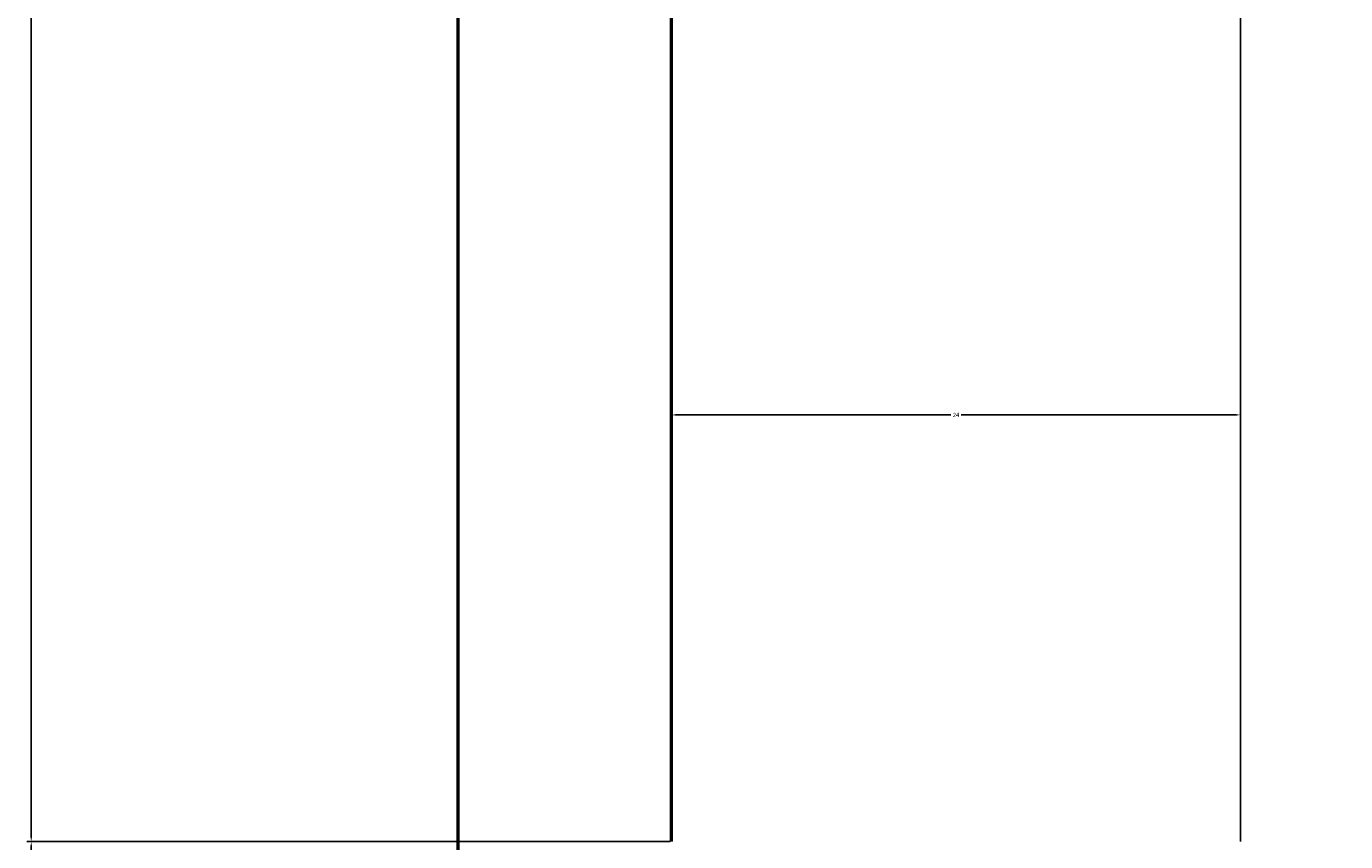
# Model space of a CAD drawing. Units: inches. Extents: x 2621 to 2849, y 2066 to 2463.
# Tile 7 of 28: x 2621 to 2676, y 2199 to 2234. Entities that reach past the tile are written whole.
import ezdxf

# ---------------------------------------------------------------- set-up
doc = ezdxf.new("R2010")
doc.units = ezdxf.units.IN
for name, color, linetype, lineweight in [('A-ANNO-DIMS', 2, 'Continuous', 18), ('A-FLOR-CASE', 9, 'Continuous', 25), ('A-WALL', 7, 'Continuous', 50)]:
    doc.layers.add(name, color=color, linetype=linetype, lineweight=lineweight)
doc.styles.get("Standard").update_dxf_attribs({"font": 'arial.ttf'})
doc.dimstyles.get("Standard").update_dxf_attribs({"dimtxt": 0.18, "dimasz": 0.18, "dimexe": 0.18, "dimexo": 0.0625, "dimgap": 0.09, "dimtad": 0, "dimtih": 1, "dimtoh": 1, "dimdec": 4, "dimzin": 0, "dimdsep": 46, "dimtxsty": 'Standard', "dimcen": 0.09, "dimadec": 0, "dimazin": 0, "dimtfac": 1, "dimtdec": 4, "dimtofl": 0, "dimtmove": 0, "dimatfit": 3, "dimfxl": 1, "dimtolj": 1, "dimtzin": 0, "dimarcsym": 0})

# ---------------------------------------------------------------- blocks, each defined once
blk = doc.blocks.new('*D56')
at = {"layer": 'A-ANNO-DIMS', "color": 0, "lineweight": -2, "transparency": 16777216}
for p, q in [((2647.87, 2199.437), (2647.87, 2217.558)), ((2648.05, 2217.378), (2659.65, 2217.378)), ((2671.69, 2217.378), (2660.09, 2217.378)), ((2671.87, 2199.437), (2671.87, 2217.558))]:
    blk.add_line(p, q, dxfattribs=at)
at = {"layer": 'A-ANNO-DIMS', "color": 0, "transparency": 16777216}
for points in [[(2648.05, 2217.408), (2648.05, 2217.348), (2647.87, 2217.378)], [(2671.69, 2217.408), (2671.69, 2217.348), (2671.87, 2217.378)]]:
    blk.add_solid(points, dxfattribs=at)
at = {"layer": 'Defpoints', "color": 0, "transparency": 16777216}
for p in [(2671.87, 2217.378), (2647.87, 2199.375), (2671.87, 2199.375)]:
    blk.add_point(p, dxfattribs=at)
at = {"layer": 'A-ANNO-DIMS', "color": 0, "transparency": 16777216, "insert": (2659.87, 2217.378), "char_height": 0.18, "attachment_point": 5}
blk.add_mtext('\\A1;24', dxfattribs=at)
blk = doc.blocks.new('*D57')
at = {"layer": 'A-ANNO-DIMS', "color": 0, "lineweight": -2, "transparency": 16777216}
for p, q in [((2647.808, 2315.375), (2620.687, 2315.375)), ((2620.867, 2315.195), (2620.867, 2257.556)), ((2620.867, 2199.555), (2620.867, 2257.193)), ((2647.808, 2199.375), (2620.687, 2199.375))]:
    blk.add_line(p, q, dxfattribs=at)
at = {"layer": 'A-ANNO-DIMS', "color": 0, "transparency": 16777216}
for points in [[(2620.837, 2315.195), (2620.897, 2315.195), (2620.867, 2315.375)], [(2620.837, 2199.555), (2620.897, 2199.555), (2620.867, 2199.375)]]:
    blk.add_solid(points, dxfattribs=at)
at = {"layer": 'Defpoints', "color": 0, "transparency": 16777216}
for p in [(2620.867, 2315.375), (2647.87, 2315.375), (2647.87, 2199.375)]:
    blk.add_point(p, dxfattribs=at)
at = {"layer": 'A-ANNO-DIMS', "color": 0, "transparency": 16777216, "insert": (2620.867, 2257.375), "char_height": 0.18, "attachment_point": 5}
blk.add_mtext('\\A1;116', dxfattribs=at)
blk = doc.blocks.new('*D62')
at = {"layer": 'A-ANNO-DIMS', "color": 0, "lineweight": -2, "transparency": 16777216}
for p, q in [((2647.808, 2199.375), (2620.687, 2199.375)), ((2620.867, 2199.195), (2620.867, 2148.556)), ((2620.867, 2097.555), (2620.867, 2148.193)), ((2647.808, 2097.375), (2620.687, 2097.375))]:
    blk.add_line(p, q, dxfattribs=at)
at = {"layer": 'A-ANNO-DIMS', "color": 0, "transparency": 16777216}
for points in [[(2620.837, 2199.195), (2620.897, 2199.195), (2620.867, 2199.375)], [(2620.837, 2097.555), (2620.897, 2097.555), (2620.867, 2097.375)]]:
    blk.add_solid(points, dxfattribs=at)
at = {"layer": 'Defpoints', "color": 0, "transparency": 16777216}
for p in [(2620.867, 2199.375), (2647.87, 2199.375), (2647.87, 2097.375)]:
    blk.add_point(p, dxfattribs=at)
at = {"layer": 'A-ANNO-DIMS', "color": 0, "transparency": 16777216, "insert": (2620.867, 2148.375), "char_height": 0.18, "attachment_point": 5}
blk.add_mtext('\\A1;102', dxfattribs=at)

msp = doc.modelspace()

# ---------------------------------------------------------------- linework, layer by layer
at = {"layer": 'A-FLOR-CASE'}
msp.add_line((2671.8701, 2199.3746), (2671.8701, 2291.3746), dxfattribs=at)
at = {"layer": 'A-WALL'}
msp.add_line((2647.8701, 2199.3746), (2647.8701, 2315.3746), dxfattribs=at)
msp.add_lwpolyline([(2761.8701, 2084.3746), (2638.8701, 2084.3746), (2638.8701, 2444.3746), (2830.8701, 2444.3746), (2830.8701, 2084.3746), (2797.8701, 2084.3746)], dxfattribs=at)

# ---------------------------------------------------------------- dimensions: what is measured, and where the dimension line sits
at = {"layer": 'A-ANNO-DIMS'}
for base, p1, p2, picture, middle in [((2620.8666, 2315.3746), (2647.8701, 2199.3746), (2647.8701, 2315.3746), '*D57', (2620.8666, 2257.3746)), ((2620.8666, 2199.3746), (2647.8701, 2097.3746), (2647.8701, 2199.3746), '*D62', (2620.8666, 2148.3746))]:
    dim = msp.add_linear_dim(base=base, p1=p1, p2=p2, angle=90, dimstyle='Standard', override={"dimdec": 0, "dimlfac": 1, "dimrnd": 0, "dimzin": 0, "dimdsep": 46, "dimlunit": 2}, dxfattribs=at)
    dim.commit()
    dim.dimension.update_dxf_attribs({"geometry": picture, "text_midpoint": middle})
dim = msp.add_linear_dim(base=(2671.8701, 2217.3781), p1=(2647.8701, 2199.3746), p2=(2671.8701, 2199.3746), dimstyle='Standard', override={"dimdec": 0, "dimlfac": 1, "dimrnd": 0, "dimzin": 0, "dimdsep": 46, "dimlunit": 2}, dxfattribs=at)
dim.commit()
dim.dimension.update_dxf_attribs({"geometry": '*D56', "text_midpoint": (2659.8701, 2217.3781)})

doc.saveas('drawing.dxf')
